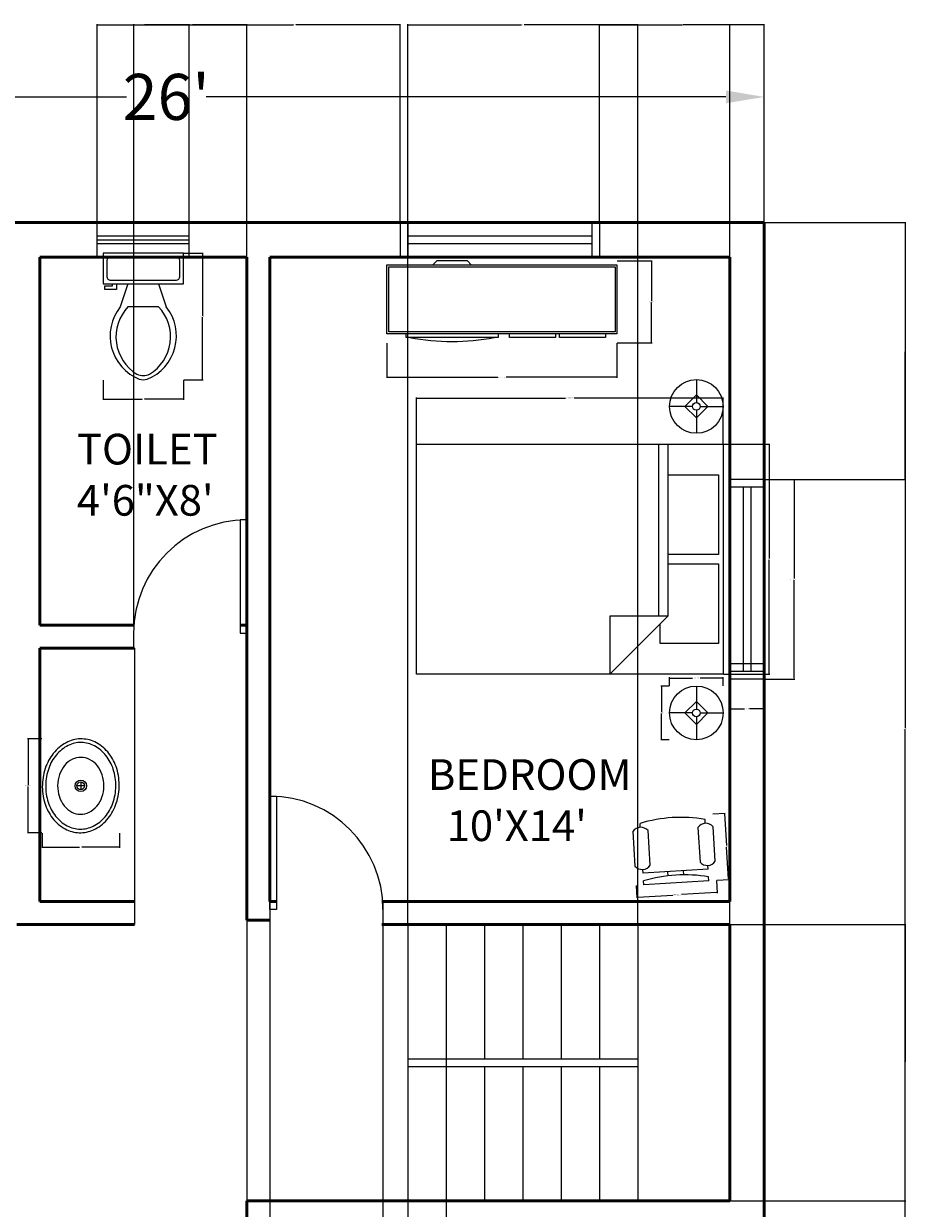
# Model space of a CAD drawing. Units: inches. Extents: x 177 to 602, y 30 to 608.
# Tile 4 of 4: x 372 to 602, y 299 to 608. Entities that reach past the tile are written whole.
import ezdxf

# ---------------------------------------------------------------- set-up
doc = ezdxf.new("R2010")
doc.units = ezdxf.units.IN
doc.header["$MEASUREMENT"] = 0
for name, color, linetype, lineweight in [('A-ANNO-DIMS', 2, 'Continuous', 18), ('A-AREA-IDEN', 7, 'Continuous', 25), ('A-DOOR', 3, 'Continuous', 25), ('A-FLOR-CASE', 32, 'Continuous', 25), ('A-FLOR-FIXT', 9, 'Continuous', 20), ('A-FLOR-STRS', 7, 'Continuous', 25), ('A-FURN', 8, 'Continuous', 18), ('A-GLAZ', 4, 'Continuous', 18), ('A-WALL', 7, 'Continuous', 50)]:
    doc.layers.add(name, color=color, linetype=linetype, lineweight=lineweight)
doc.styles.get("Standard").update_dxf_attribs({"font": 'arial.ttf'})
doc.dimstyles.get("Standard").update_dxf_attribs({"dimtxt": 0.18, "dimasz": 0.18, "dimexe": 0.18, "dimexo": 0.0625, "dimgap": 0.09, "dimtad": 0, "dimtih": 1, "dimtoh": 1, "dimdec": 1, "dimzin": 0, "dimdsep": 46, "dimlunit": 4, "dimtxsty": 'Standard', "dimcen": 0.09, "dimadec": 0, "dimazin": 0, "dimtfac": 1, "dimtdec": 1, "dimtofl": 0, "dimtmove": 0, "dimatfit": 3, "dimfxl": 1, "dimtolj": 1, "dimtzin": 0, "dimarcsym": 0})

# ---------------------------------------------------------------- blocks, each defined once
blk = doc.blocks.new('*U16')
for p, q in [((-750, 0), (-750, -100)), ((0, 0), (0, -100))]:
    blk.add_line(p, q)
blk.add_lwpolyline([(0, 0), (0, 750), (-43.75, 750), (-43.75, 0)], close=True)
blk.add_arc((0, 0), 750, 90, 180)
blk = doc.blocks.new('Toilet - top')
for p, q in [((9.5, -6), (9.5, -2)), ((-10, -8.5), (-8, -8.5)), ((-10, -9.5), (-10, -8.5)), ((-8, -8.5), (-8, -8)), ((-7, -8), (-7, -9.5)), ((-4, -8), (-6, -14)), ((4, -8), (6, -14)), ((-7, -9.5), (-10, -9.5)), ((4, -14), (-4, -14))]:
    blk.add_line(p, q)
blk.add_lwpolyline([(10.5, -8), (10.5, 0), (-10.5, 0), (-10.5, -8)], close=True)
for points in [[(-9.5, -2), (-9.5, -6)], [(8.5, -1), (-8.5, -1)], [(-8.5, -7), (8.5, -7)]]:
    blk.add_lwpolyline(points)
for centre, radius, start, end in [((-8.62, -1.88), 0.884, 81.8699, 188.1301), ((8.62, -1.88), 0.884, 351.8699, 98.1301), ((-8.62, -6.12), 0.884, 171.8699, 278.1301), ((8.62, -6.12), 0.884, 261.8699, 8.1301), ((3.52, -21.58), 12.17, 141.4691, 247.9714), ((4.2, -21.82), 11.33, 136.3677, 238.9468), ((-3.52, -21.58), 12.17, 292.0284, 38.5307), ((-4.2, -21.82), 11.33, 301.053, 43.6321), ((0, -27.88), 4, 245.7318, 294.2682), ((0, -29), 4, 254.8605, 285.1395)]:
    blk.add_arc(centre, radius, start, end)
blk = doc.blocks.new('Sink - Oval top')
for p, q in [((-1, 0), (1, 0)), ((0, 1), (0, -1))]:
    blk.add_line(p, q)
for points in [[(-12.23, 0.39, 0.117634), (-11.46, -3.36, 0.104469), (-8.88, -6.8, 0.090016), (-5.08, -9.07, 0.08192), (-0.32, -10.02, 0.08192), (4.49, -9.38, 0.090016), (8.42, -7.36, 0.104469), (11.22, -4.09, 0.117634), (12.23, -0.39, 0.117634), (11.46, 3.36, 0.104469), (8.88, 6.8, 0.090016), (5.08, 9.07, 0.08192), (0.32, 10.02, 0.08192), (-4.49, 9.38, 0.090016), (-8.42, 7.36, 0.104469), (-11.22, 4.09, 0.117634)], [(-11.29, 0.16, 0.118622), (-10.52, -3.25, 0.104678), (-8.07, -6.36, 0.089562), (-4.54, -8.37, 0.081185), (-0.13, -9.15, 0.081185), (4.3, -8.49, 0.089562), (7.89, -6.58, 0.104678), (10.42, -3.55, 0.118622), (11.29, -0.16, 0.118622), (10.52, 3.25, 0.104678), (8.07, 6.36, 0.089562), (4.54, 8.37, 0.081185), (0.13, 9.15, 0.081185), (-4.3, 8.49, 0.089562), (-7.89, 6.58, 0.104678), (-10.42, 3.55, 0.118622)], [(-7.42, 0.08, 0.118283), (-6.91, -2.17, 0.104607), (-5.29, -4.21, 0.089718), (-2.97, -5.53, 0.081436), (-0.07, -6.04, 0.081436), (2.84, -5.59, 0.089718), (5.2, -4.33, 0.104607), (6.86, -2.32, 0.118283), (7.42, -0.08, 0.118283), (6.91, 2.17, 0.104607), (5.29, 4.21, 0.089718), (2.97, 5.53, 0.081436), (0.07, 6.04, 0.081436), (-2.84, 5.59, 0.089718), (-5.2, 4.33, 0.104607), (-6.86, 2.32, 0.118283)]]:
    blk.add_lwpolyline(points, format="xyb", close=True)
for radius in [1.5, 1]:
    blk.add_circle((0, 0), radius)
blk = doc.blocks.new('*U2')
for p, q in [((0, 0), (0, -100)), ((750, 0), (750, -100))]:
    blk.add_line(p, q)
blk.add_lwpolyline([(0, 0), (0, 750), (43.75, 750), (43.75, 0)], close=True)
blk.add_arc((0, 0), 750, 0, 90)
blk = doc.blocks.new('Bed - Queen')
for p, q in [((0, -80.00003), (0, 0)), ((0, 0), (59.99999, 0)), ((59.99999, 0), (59.99999, -80.00003)), ((7.99999, -1.2), (28.79998, -1.2)), ((7.99999, -14.4), (7.99999, -1.2)), ((28.79998, -1.2), (28.79998, -14.4)), ((31.19999, -1.2), (51.99999, -1.2)), ((31.19999, -14.4), (31.19999, -1.2)), ((51.99999, -1.2), (51.99999, -16.4)), ((0, -14.4), (44.8, -14.4)), ((59.99999, -29.6), (44.8, -14.4)), ((44.8, -14.4), (44.8, -29.6)), ((44.8, -16.8), (0, -16.8)), ((51.99999, -16.4), (46.79936, -16.4)), ((44.8, -29.6), (59.99999, -29.6)), ((59.99999, -80.00003), (0, -80.00003))]:
    blk.add_line(p, q)
blk = doc.blocks.new('Lamp - Table')
for p, q in [((0, 7), (0, 1)), ((-1, 0), (-7, 0)), ((0, 3), (-3, 0)), ((-3, 0), (0, -3)), ((3, 0), (0, 3)), ((0, -3), (3, 0)), ((1, 0), (7, 0)), ((0, -1), (0, -7))]:
    blk.add_line(p, q)
for radius in [7, 1]:
    blk.add_circle((0, 0), radius)
blk = doc.blocks.new('Entertainment Center')
for p, q in [((-4, 0), (-5, -1)), ((4, 0), (-4, 0)), ((5, -1), (4, 0)), ((-17, -19), (-17, -1)), ((-17, -1), (43, -1)), ((-16.5, -18.5), (-16.5, -1.5)), ((-16.5, -1.5), (42.5, -1.5)), ((42.5, -1.5), (42.5, -18.5)), ((43, -1), (43, -19)), ((42.5, -18.5), (-16.5, -18.5)), ((43, -19), (-17, -19)), ((-12, -20), (-12, -19)), ((12, -20), (-12, -20)), ((12, -19), (12, -20)), ((15, -20), (15, -19)), ((27, -20), (15, -20)), ((27, -19), (27, -20)), ((28, -20), (28, -19)), ((40, -20), (28, -20)), ((40, -19), (40, -20))]:
    blk.add_line(p, q)
blk.add_arc((0, 40), 61, 259.6111, 280.3889)
blk = doc.blocks.new('Chair - Desk')
for p, q in [((-8.5, 0), (-8.5, -1)), ((-8.5, 0), (8.5, 0)), ((8.5, 0), (8.5, -1)), ((-8.5, -3), (-8.5, -4)), ((-8.5, -3), (8.5, -3)), ((-2, -3), (-2, -1.9355)), ((2, -1.9576), (2, -3)), ((8.5, -3), (8.5, -4)), ((-10.5, -5), (-10.5, -14)), ((-6.5, -14), (-6.5, -5)), ((6.5, -5), (6.5, -14)), ((10.5, -14), (10.5, -5)), ((-8.5, -15), (-8.5, -16)), ((8.5, -15), (8.5, -16))]:
    blk.add_line(p, q)
for centre, radius, start, end in [((0, 34.625), 36.625, 256.5803, 283.4197), ((-8.5, -6.5), 2.5, 36.8699, 143.1301), ((8.5, -6.5), 2.5, 36.8699, 143.1301), ((-8.5, -12.5), 2.5, 216.8699, 323.1301), ((8.5, -12.5), 2.5, 216.8699, 323.1301), ((0, 19.625), 36.625, 256.5803, 283.4197)]:
    blk.add_arc(centre, radius, start, end)
blk = doc.blocks.new('*D32')
at = {"layer": 'A-ANNO-DIMS', "color": 0, "lineweight": -2, "transparency": 16777216}
for p, q in [((253.34, 556.2), (253.34, 589.06)), ((263.34, 588.88), (398.96, 588.88)), ((555.34, 588.88), (419.71, 588.88)), ((565.34, 556.2), (565.34, 589.06))]:
    blk.add_line(p, q, dxfattribs=at)
at = {"layer": 'A-ANNO-DIMS', "color": 0, "transparency": 16777216}
for points in [[(263.34, 590.55), (263.34, 587.22), (253.34, 588.88)], [(555.34, 590.55), (555.34, 587.22), (565.34, 588.88)]]:
    blk.add_solid(points, dxfattribs=at)
at = {"layer": 'Defpoints', "color": 0, "transparency": 16777216}
for p in [(565.34, 588.88), (253.34, 556.14), (565.34, 556.14)]:
    blk.add_point(p, dxfattribs=at)
at = {"layer": 'A-ANNO-DIMS', "color": 0, "transparency": 16777216, "insert": (409.34, 588.88), "char_height": 12, "attachment_point": 5}
blk.add_mtext("\\A1;26'", dxfattribs=at)
blk = doc.blocks.new('WIN-48IN')
for p, q in [((9, 52), (0, 52)), ((9, 50), (0, 50)), ((3.5, 50), (3.5, 2)), ((5.5, 50), (5.5, 2)), ((9, 2), (0, 2)), ((9, 0), (0, 0))]:
    blk.add_line(p, q)
blk = doc.blocks.new('*D37')
at = {"layer": 'A-ANNO-DIMS', "color": 0, "lineweight": -2, "transparency": 16777216}
for p, q in [((565.4, 489.14), (573.32, 489.14)), ((573.14, 488.96), (573.14, 463.32)), ((573.14, 437.32), (573.14, 462.95)), ((565.4, 437.14), (573.32, 437.14))]:
    blk.add_line(p, q, dxfattribs=at)
at = {"layer": 'A-ANNO-DIMS', "color": 0, "transparency": 16777216}
for points in [[(573.11, 488.96), (573.17, 488.96), (573.14, 489.14)], [(573.11, 437.32), (573.17, 437.32), (573.14, 437.14)]]:
    blk.add_solid(points, dxfattribs=at)
at = {"layer": 'Defpoints', "color": 0, "transparency": 16777216}
for p in [(565.34, 489.14), (573.14, 489.14), (565.34, 437.14)]:
    blk.add_point(p, dxfattribs=at)
at = {"layer": 'A-ANNO-DIMS', "color": 0, "transparency": 16777216, "insert": (573.14, 463.14), "char_height": 0.18, "attachment_point": 5}
blk.add_mtext('\\A1;WINDOW 4\'-4" TYP.', dxfattribs=at)
blk = doc.blocks.new('*D38')
at = {"layer": 'A-ANNO-DIMS', "color": 0, "lineweight": -2, "transparency": 16777216}
for p, q in [((556.34, 437.07), (556.34, 429.16)), ((565.34, 437.07), (565.34, 429.16)), ((556.52, 429.34), (560.2, 429.34)), ((565.16, 429.34), (561.48, 429.34))]:
    blk.add_line(p, q, dxfattribs=at)
at = {"layer": 'A-ANNO-DIMS', "color": 0, "transparency": 16777216}
for points in [[(556.52, 429.37), (556.52, 429.31), (556.34, 429.34)], [(565.16, 429.37), (565.16, 429.31), (565.34, 429.34)]]:
    blk.add_solid(points, dxfattribs=at)
at = {"layer": 'Defpoints', "color": 0, "transparency": 16777216}
for p in [(556.34, 437.14), (565.34, 437.14), (565.34, 429.34)]:
    blk.add_point(p, dxfattribs=at)
at = {"layer": 'A-ANNO-DIMS', "color": 0, "transparency": 16777216, "insert": (560.84, 429.34), "char_height": 0.18, "attachment_point": 5}
blk.add_mtext('\\A1;0\'-9" TYP.', dxfattribs=at)
blk = doc.blocks.new('*D39')
at = {"layer": 'A-ANNO-DIMS', "color": 0, "lineweight": -2, "transparency": 16777216}
for p, q in [((540.61, 435.37), (540.61, 437.58)), ((540.79, 437.4), (546.6, 437.4)), ((554.43, 437.4), (548.62, 437.4)), ((554.61, 435.37), (554.61, 437.58))]:
    blk.add_line(p, q, dxfattribs=at)
at = {"layer": 'A-ANNO-DIMS', "color": 0, "transparency": 16777216}
for points in [[(540.79, 437.43), (540.79, 437.37), (540.61, 437.4)], [(554.43, 437.43), (554.43, 437.37), (554.61, 437.4)]]:
    blk.add_solid(points, dxfattribs=at)
at = {"layer": 'Defpoints', "color": 0, "transparency": 16777216}
for p in [(554.61, 437.4), (540.61, 435.3), (554.61, 435.3)]:
    blk.add_point(p, dxfattribs=at)
at = {"layer": 'A-ANNO-DIMS', "color": 0, "transparency": 16777216, "insert": (547.61, 437.4), "char_height": 0.18, "attachment_point": 5}
blk.add_mtext('\\A1;LAMP 1\'-2" TYP.', dxfattribs=at)
blk = doc.blocks.new('*D40')
at = {"layer": 'A-ANNO-DIMS', "color": 0, "lineweight": -2, "transparency": 16777216}
for p, q in [((540.55, 435.3), (538.33, 435.3)), ((538.51, 435.12), (538.51, 428.48)), ((538.51, 421.48), (538.51, 428.12)), ((540.55, 421.3), (538.33, 421.3))]:
    blk.add_line(p, q, dxfattribs=at)
at = {"layer": 'A-ANNO-DIMS', "color": 0, "transparency": 16777216}
for points in [[(538.48, 435.12), (538.54, 435.12), (538.51, 435.3)], [(538.48, 421.48), (538.54, 421.48), (538.51, 421.3)]]:
    blk.add_solid(points, dxfattribs=at)
at = {"layer": 'Defpoints', "color": 0, "transparency": 16777216}
for p in [(538.51, 435.3), (540.61, 435.3), (540.61, 421.3)]:
    blk.add_point(p, dxfattribs=at)
at = {"layer": 'A-ANNO-DIMS', "color": 0, "transparency": 16777216, "insert": (538.51, 428.3), "char_height": 0.18, "attachment_point": 5}
blk.add_mtext('\\A1;1\'-2" TYP.', dxfattribs=at)
blk = doc.blocks.new('*D49')
at = {"layer": 'A-ANNO-DIMS', "color": 0, "lineweight": -2, "transparency": 16777216}
for p, q in [((413.9, 548.14), (418.98, 548.14)), ((418.8, 547.96), (418.8, 531.8)), ((418.8, 515.27), (418.8, 531.43)), ((413.9, 515.09), (418.98, 515.09))]:
    blk.add_line(p, q, dxfattribs=at)
at = {"layer": 'A-ANNO-DIMS', "color": 0, "transparency": 16777216}
for points in [[(418.77, 547.96), (418.83, 547.96), (418.8, 548.14)], [(418.77, 515.27), (418.83, 515.27), (418.8, 515.09)]]:
    blk.add_solid(points, dxfattribs=at)
at = {"layer": 'Defpoints', "color": 0, "transparency": 16777216}
for p in [(413.84, 548.14), (418.8, 548.14), (413.84, 515.09)]:
    blk.add_point(p, dxfattribs=at)
at = {"layer": 'A-ANNO-DIMS', "color": 0, "transparency": 16777216, "insert": (418.8, 531.61), "char_height": 0.18, "attachment_point": 5}
blk.add_mtext('\\A1;WC 2\'-9"', dxfattribs=at)
blk = doc.blocks.new('*D50')
at = {"layer": 'A-ANNO-DIMS', "color": 0, "lineweight": -2, "transparency": 16777216}
for p, q in [((392.84, 515.03), (392.84, 509.95)), ((413.84, 515.03), (413.84, 509.95)), ((393.02, 510.13), (403.02, 510.13)), ((413.66, 510.13), (403.66, 510.13))]:
    blk.add_line(p, q, dxfattribs=at)
at = {"layer": 'A-ANNO-DIMS', "color": 0, "transparency": 16777216}
for points in [[(393.02, 510.16), (393.02, 510.1), (392.84, 510.13)], [(413.66, 510.16), (413.66, 510.1), (413.84, 510.13)]]:
    blk.add_solid(points, dxfattribs=at)
at = {"layer": 'Defpoints', "color": 0, "transparency": 16777216}
for p in [(392.84, 515.09), (413.84, 515.09), (413.84, 510.13)]:
    blk.add_point(p, dxfattribs=at)
at = {"layer": 'A-ANNO-DIMS', "color": 0, "transparency": 16777216, "insert": (403.34, 510.13), "char_height": 0.18, "attachment_point": 5}
blk.add_mtext('\\A1;1\'-9"', dxfattribs=at)
blk = doc.blocks.new('*D51')
at = {"layer": 'A-ANNO-DIMS', "color": 0, "lineweight": -2, "transparency": 16777216}
for p, q in [((376.9, 421.58), (373.1, 421.58)), ((373.28, 421.4), (373.28, 409.48)), ((373.28, 397.21), (373.28, 409.12)), ((376.9, 397.03), (373.1, 397.03))]:
    blk.add_line(p, q, dxfattribs=at)
at = {"layer": 'A-ANNO-DIMS', "color": 0, "transparency": 16777216}
for points in [[(373.25, 421.4), (373.31, 421.4), (373.28, 421.58)], [(373.25, 397.21), (373.31, 397.21), (373.28, 397.03)]]:
    blk.add_solid(points, dxfattribs=at)
at = {"layer": 'Defpoints', "color": 0, "transparency": 16777216}
for p in [(376.96, 421.58), (373.28, 397.03), (376.96, 397.03)]:
    blk.add_point(p, dxfattribs=at)
at = {"layer": 'A-ANNO-DIMS', "color": 0, "transparency": 16777216, "insert": (373.28, 409.3), "char_height": 0.18, "attachment_point": 5}
blk.add_mtext('\\A1;BASIN 2\'-0 1/2"', dxfattribs=at)
blk = doc.blocks.new('*D52')
at = {"layer": 'A-ANNO-DIMS', "color": 0, "lineweight": -2, "transparency": 16777216}
for p, q in [((376.96, 396.96), (376.96, 393.16)), ((397.1, 396.96), (397.1, 393.16)), ((377.14, 393.34), (386.71, 393.34)), ((396.92, 393.34), (387.35, 393.34))]:
    blk.add_line(p, q, dxfattribs=at)
at = {"layer": 'A-ANNO-DIMS', "color": 0, "transparency": 16777216}
for points in [[(377.14, 393.37), (377.14, 393.31), (376.96, 393.34)], [(396.92, 393.37), (396.92, 393.31), (397.1, 393.34)]]:
    blk.add_solid(points, dxfattribs=at)
at = {"layer": 'Defpoints', "color": 0, "transparency": 16777216}
for p in [(376.96, 397.03), (397.1, 397.03), (397.1, 393.34)]:
    blk.add_point(p, dxfattribs=at)
at = {"layer": 'A-ANNO-DIMS', "color": 0, "transparency": 16777216, "insert": (387.03, 393.34), "char_height": 0.18, "attachment_point": 5}
blk.add_mtext('\\A1;1\'-8"', dxfattribs=at)
blk = doc.blocks.new('*D53')
at = {"layer": 'A-ANNO-DIMS', "color": 0, "lineweight": -2, "transparency": 16777216}
for p, q in [((474.61, 498.42), (474.61, 510.54)), ((474.79, 510.36), (513.5, 510.36)), ((554.43, 510.36), (515.71, 510.36)), ((554.61, 498.42), (554.61, 510.54))]:
    blk.add_line(p, q, dxfattribs=at)
at = {"layer": 'A-ANNO-DIMS', "color": 0, "transparency": 16777216}
for points in [[(474.79, 510.39), (474.79, 510.33), (474.61, 510.36)], [(554.43, 510.39), (554.43, 510.33), (554.61, 510.36)]]:
    blk.add_solid(points, dxfattribs=at)
at = {"layer": 'Defpoints', "color": 0, "transparency": 16777216}
for p in [(554.61, 510.36), (474.61, 498.36), (554.61, 498.36)]:
    blk.add_point(p, dxfattribs=at)
at = {"layer": 'A-ANNO-DIMS', "color": 0, "transparency": 16777216, "insert": (514.61, 510.36), "char_height": 0.18, "attachment_point": 5}
blk.add_mtext('\\A1;QUEEN BED 6\'-8"', dxfattribs=at)
blk = doc.blocks.new('*D54')
at = {"layer": 'A-ANNO-DIMS', "color": 0, "lineweight": -2, "transparency": 16777216}
for p, q in [((554.67, 498.36), (566.79, 498.36)), ((566.61, 498.18), (566.61, 468.54)), ((566.61, 438.54), (566.61, 468.18)), ((554.67, 438.36), (566.79, 438.36))]:
    blk.add_line(p, q, dxfattribs=at)
at = {"layer": 'A-ANNO-DIMS', "color": 0, "transparency": 16777216}
for points in [[(566.58, 498.18), (566.64, 498.18), (566.61, 498.36)], [(566.58, 438.54), (566.64, 438.54), (566.61, 438.36)]]:
    blk.add_solid(points, dxfattribs=at)
at = {"layer": 'Defpoints', "color": 0, "transparency": 16777216}
for p in [(554.61, 498.36), (554.61, 438.36), (566.61, 438.36)]:
    blk.add_point(p, dxfattribs=at)
at = {"layer": 'A-ANNO-DIMS', "color": 0, "transparency": 16777216, "insert": (566.61, 468.36), "char_height": 0.18, "attachment_point": 5}
blk.add_mtext('\\A1;5\'-0"', dxfattribs=at)
blk = doc.blocks.new('*D55')
at = {"layer": 'A-ANNO-DIMS', "color": 0, "lineweight": -2, "transparency": 16777216}
for p, q in [((466.89, 524.73), (466.89, 515.61)), ((526.89, 524.73), (526.89, 515.61)), ((467.07, 515.79), (495.81, 515.79)), ((526.71, 515.79), (497.98, 515.79))]:
    blk.add_line(p, q, dxfattribs=at)
at = {"layer": 'A-ANNO-DIMS', "color": 0, "transparency": 16777216}
for points in [[(467.07, 515.82), (467.07, 515.76), (466.89, 515.79)], [(526.71, 515.82), (526.71, 515.76), (526.89, 515.79)]]:
    blk.add_solid(points, dxfattribs=at)
at = {"layer": 'Defpoints', "color": 0, "transparency": 16777216}
for p in [(466.89, 524.79), (526.89, 524.79), (526.89, 515.79)]:
    blk.add_point(p, dxfattribs=at)
at = {"layer": 'A-ANNO-DIMS', "color": 0, "transparency": 16777216, "insert": (496.89, 515.79), "char_height": 0.18, "attachment_point": 5}
blk.add_mtext('\\A1;MEDIA UNIT 5\'-0"', dxfattribs=at)
blk = doc.blocks.new('*D56')
at = {"layer": 'A-ANNO-DIMS', "color": 0, "lineweight": -2, "transparency": 16777216}
for p, q in [((526.96, 546.13), (536.07, 546.13)), ((535.89, 545.95), (535.89, 535.64)), ((535.89, 524.97), (535.89, 535.28)), ((526.96, 524.79), (536.07, 524.79))]:
    blk.add_line(p, q, dxfattribs=at)
at = {"layer": 'A-ANNO-DIMS', "color": 0, "transparency": 16777216}
for points in [[(535.86, 545.95), (535.92, 545.95), (535.89, 546.13)], [(535.86, 524.97), (535.92, 524.97), (535.89, 524.79)]]:
    blk.add_solid(points, dxfattribs=at)
at = {"layer": 'Defpoints', "color": 0, "transparency": 16777216}
for p in [(526.89, 546.13), (535.89, 546.13), (526.89, 524.79)]:
    blk.add_point(p, dxfattribs=at)
at = {"layer": 'A-ANNO-DIMS', "color": 0, "transparency": 16777216, "insert": (535.89, 535.46), "char_height": 0.18, "attachment_point": 5}
blk.add_mtext('\\A1;1\'-9 1/2"', dxfattribs=at)
blk = doc.blocks.new('*D63')
at = {"layer": 'A-ANNO-DIMS', "color": 0, "lineweight": -2, "transparency": 16777216}
for p, q in [((531.91, 383.32), (532.11, 380.06)), ((552.87, 384.61), (553.07, 381.35)), ((532.28, 380.25), (541.45, 380.82)), ((552.88, 381.52), (543.7, 380.95))]:
    blk.add_line(p, q, dxfattribs=at)
at = {"layer": 'A-ANNO-DIMS', "color": 0, "transparency": 16777216}
for points in [[(532.27, 380.28), (532.28, 380.22), (532.1, 380.24)], [(552.88, 381.55), (552.88, 381.49), (553.06, 381.53)]]:
    blk.add_solid(points, dxfattribs=at)
at = {"layer": 'Defpoints', "color": 0, "transparency": 16777216}
for p in [(531.9, 383.39), (552.86, 384.67), (532.1, 380.24)]:
    blk.add_point(p, dxfattribs=at)
at = {"layer": 'A-ANNO-DIMS', "color": 0, "transparency": 16777216, "insert": (542.58, 380.88), "char_height": 0.18, "attachment_point": 5}
blk.add_mtext('\\A1;DESK CHAIR 1\'-9"', dxfattribs=at)
blk = doc.blocks.new('*D64')
at = {"layer": 'A-ANNO-DIMS', "color": 0, "lineweight": -2, "transparency": 16777216}
for p, q in [((551.87, 401.98), (555.13, 402.18)), ((554.96, 401.98), (555.47, 393.7)), ((556, 385.04), (555.49, 393.33)), ((552.93, 384.67), (556.19, 384.87))]:
    blk.add_line(p, q, dxfattribs=at)
at = {"layer": 'A-ANNO-DIMS', "color": 0, "transparency": 16777216}
for points in [[(554.99, 401.99), (554.93, 401.98), (554.95, 402.16)], [(556.03, 385.04), (555.97, 385.04), (556.01, 384.86)]]:
    blk.add_solid(points, dxfattribs=at)
at = {"layer": 'Defpoints', "color": 0, "transparency": 16777216}
for p in [(551.8, 401.97), (552.86, 384.67), (556.01, 384.86)]:
    blk.add_point(p, dxfattribs=at)
at = {"layer": 'A-ANNO-DIMS', "color": 0, "transparency": 16777216, "insert": (555.48, 393.51), "char_height": 0.18, "attachment_point": 5}
blk.add_mtext('\\A1;1\'-5 1/2"', dxfattribs=at)
blk = doc.blocks.new('*D74')
at = {"layer": 'A-ANNO-DIMS', "color": 0, "lineweight": -2, "transparency": 16777216}
for p, q in [((565.4, 556.14), (602.22, 556.14)), ((602.04, 555.96), (602.04, 424.32)), ((602.04, 292.32), (602.04, 423.96)), ((565.4, 292.14), (602.22, 292.14))]:
    blk.add_line(p, q, dxfattribs=at)
at = {"layer": 'A-ANNO-DIMS', "color": 0, "transparency": 16777216}
for points in [[(602.01, 555.96), (602.07, 555.96), (602.04, 556.14)], [(602.01, 292.32), (602.07, 292.32), (602.04, 292.14)]]:
    blk.add_solid(points, dxfattribs=at)
at = {"layer": 'Defpoints', "color": 0, "transparency": 16777216}
for p in [(565.34, 556.14), (602.04, 556.14), (565.34, 292.14)]:
    blk.add_point(p, dxfattribs=at)
at = {"layer": 'A-ANNO-DIMS', "color": 0, "transparency": 16777216, "insert": (602.04, 424.14), "char_height": 0.18, "attachment_point": 5}
blk.add_mtext('\\A1;22\'-0"', dxfattribs=at)
blk = doc.blocks.new('*D79')
at = {"layer": 'A-ANNO-DIMS', "color": 0, "lineweight": -2, "transparency": 16777216}
for p, q in [((522.34, 556.2), (522.34, 607.88)), ((522.52, 607.7), (543.51, 607.7)), ((565.16, 607.7), (544.17, 607.7)), ((565.34, 556.2), (565.34, 607.88))]:
    blk.add_line(p, q, dxfattribs=at)
at = {"layer": 'A-ANNO-DIMS', "color": 0, "transparency": 16777216}
for points in [[(522.52, 607.73), (522.52, 607.67), (522.34, 607.7)], [(565.16, 607.73), (565.16, 607.67), (565.34, 607.7)]]:
    blk.add_solid(points, dxfattribs=at)
at = {"layer": 'Defpoints', "color": 0, "transparency": 16777216}
for p in [(565.34, 607.7), (522.34, 556.14), (565.34, 556.14)]:
    blk.add_point(p, dxfattribs=at)
at = {"layer": 'A-ANNO-DIMS', "color": 0, "transparency": 16777216, "insert": (543.84, 607.7), "char_height": 0.18, "attachment_point": 5}
blk.add_mtext('\\A1;3\'-7"', dxfattribs=at)
blk = doc.blocks.new('*D80')
at = {"layer": 'A-ANNO-DIMS', "color": 0, "lineweight": -2, "transparency": 16777216}
for p, q in [((565.4, 556.14), (602.22, 556.14)), ((602.04, 555.96), (602.04, 522.82)), ((602.04, 489.32), (602.04, 522.46)), ((565.4, 489.14), (602.22, 489.14))]:
    blk.add_line(p, q, dxfattribs=at)
at = {"layer": 'A-ANNO-DIMS', "color": 0, "transparency": 16777216}
for points in [[(602.01, 555.96), (602.07, 555.96), (602.04, 556.14)], [(602.01, 489.32), (602.07, 489.32), (602.04, 489.14)]]:
    blk.add_solid(points, dxfattribs=at)
at = {"layer": 'Defpoints', "color": 0, "transparency": 16777216}
for p in [(565.34, 556.14), (602.04, 556.14), (565.34, 489.14)]:
    blk.add_point(p, dxfattribs=at)
at = {"layer": 'A-ANNO-DIMS', "color": 0, "transparency": 16777216, "insert": (602.04, 522.64), "char_height": 0.18, "attachment_point": 5}
blk.add_mtext('\\A1;5\'-7"', dxfattribs=at)
blk = doc.blocks.new('*D82')
at = {"layer": 'A-ANNO-DIMS', "color": 0, "lineweight": -2, "transparency": 16777216}
for p, q in [((391.34, 556.2), (391.34, 607.88)), ((391.52, 607.7), (403.01, 607.7)), ((415.16, 607.7), (403.67, 607.7)), ((415.34, 556.2), (415.34, 607.88))]:
    blk.add_line(p, q, dxfattribs=at)
at = {"layer": 'A-ANNO-DIMS', "color": 0, "transparency": 16777216}
for points in [[(391.52, 607.73), (391.52, 607.67), (391.34, 607.7)], [(415.16, 607.73), (415.16, 607.67), (415.34, 607.7)]]:
    blk.add_solid(points, dxfattribs=at)
at = {"layer": 'Defpoints', "color": 0, "transparency": 16777216}
for p in [(415.34, 607.7), (391.34, 556.14), (415.34, 556.14)]:
    blk.add_point(p, dxfattribs=at)
at = {"layer": 'A-ANNO-DIMS', "color": 0, "transparency": 16777216, "insert": (403.34, 607.7), "char_height": 0.18, "attachment_point": 5}
blk.add_mtext('\\A1;2\'-0"', dxfattribs=at)
blk = doc.blocks.new('*D83')
at = {"layer": 'A-ANNO-DIMS', "color": 0, "lineweight": -2, "transparency": 16777216}
for p, q in [((415.34, 556.2), (415.34, 607.88)), ((415.52, 607.7), (442.51, 607.7)), ((470.16, 607.7), (443.17, 607.7)), ((470.34, 556.2), (470.34, 607.88))]:
    blk.add_line(p, q, dxfattribs=at)
at = {"layer": 'A-ANNO-DIMS', "color": 0, "transparency": 16777216}
for points in [[(415.52, 607.73), (415.52, 607.67), (415.34, 607.7)], [(470.16, 607.73), (470.16, 607.67), (470.34, 607.7)]]:
    blk.add_solid(points, dxfattribs=at)
at = {"layer": 'Defpoints', "color": 0, "transparency": 16777216}
for p in [(470.34, 607.7), (415.34, 556.14), (470.34, 556.14)]:
    blk.add_point(p, dxfattribs=at)
at = {"layer": 'A-ANNO-DIMS', "color": 0, "transparency": 16777216, "insert": (442.84, 607.7), "char_height": 0.18, "attachment_point": 5}
blk.add_mtext('\\A1;4\'-7"', dxfattribs=at)
blk = doc.blocks.new('*D84')
at = {"layer": 'A-ANNO-DIMS', "color": 0, "lineweight": -2, "transparency": 16777216}
for p, q in [((436.34, 379.07), (436.34, 30.54)), ((430.34, 374.22), (430.34, 30.54)), ((430.52, 30.72), (433.01, 30.72)), ((436.16, 30.72), (433.67, 30.72))]:
    blk.add_line(p, q, dxfattribs=at)
at = {"layer": 'A-ANNO-DIMS', "color": 0, "transparency": 16777216}
for points in [[(430.52, 30.75), (430.52, 30.69), (430.34, 30.72)], [(436.16, 30.75), (436.16, 30.69), (436.34, 30.72)]]:
    blk.add_solid(points, dxfattribs=at)
at = {"layer": 'Defpoints', "color": 0, "transparency": 16777216}
for p in [(436.34, 379.14), (430.34, 374.28), (430.34, 30.72)]:
    blk.add_point(p, dxfattribs=at)
at = {"layer": 'A-ANNO-DIMS', "color": 0, "transparency": 16777216, "insert": (433.34, 30.72), "char_height": 0.18, "attachment_point": 5}
blk.add_mtext('\\A1;0\'-6"', dxfattribs=at)
blk = doc.blocks.new('*D87')
at = {"layer": 'A-ANNO-DIMS', "color": 0, "lineweight": -2, "transparency": 16777216}
for p, q in [((436.34, 379.07), (436.34, 30.54)), ((465.79, 379.07), (465.79, 30.54)), ((436.52, 30.72), (450.53, 30.72)), ((465.61, 30.72), (451.61, 30.72))]:
    blk.add_line(p, q, dxfattribs=at)
at = {"layer": 'A-ANNO-DIMS', "color": 0, "transparency": 16777216}
for points in [[(436.52, 30.75), (436.52, 30.69), (436.34, 30.72)], [(465.61, 30.75), (465.61, 30.69), (465.79, 30.72)]]:
    blk.add_solid(points, dxfattribs=at)
at = {"layer": 'Defpoints', "color": 0, "transparency": 16777216}
for p in [(436.34, 379.14), (465.79, 379.14), (465.79, 30.72)]:
    blk.add_point(p, dxfattribs=at)
at = {"layer": 'A-ANNO-DIMS', "color": 0, "transparency": 16777216, "insert": (451.07, 30.72), "char_height": 0.18, "attachment_point": 5}
blk.add_mtext('\\A1;2\'-5 1/2"', dxfattribs=at)
blk = doc.blocks.new('*D88')
at = {"layer": 'A-ANNO-DIMS', "color": 0, "lineweight": -2, "transparency": 16777216}
for p, q in [((400.88, 451.2), (400.88, 607.88)), ((401.06, 607.7), (415.07, 607.7)), ((430.16, 607.7), (416.15, 607.7)), ((430.34, 451.2), (430.34, 607.88))]:
    blk.add_line(p, q, dxfattribs=at)
at = {"layer": 'A-ANNO-DIMS', "color": 0, "transparency": 16777216}
for points in [[(401.06, 607.73), (401.06, 607.67), (400.88, 607.7)], [(430.16, 607.73), (430.16, 607.67), (430.34, 607.7)]]:
    blk.add_solid(points, dxfattribs=at)
at = {"layer": 'Defpoints', "color": 0, "transparency": 16777216}
for p in [(430.34, 607.7), (400.88, 451.14), (430.34, 451.14)]:
    blk.add_point(p, dxfattribs=at)
at = {"layer": 'A-ANNO-DIMS', "color": 0, "transparency": 16777216, "insert": (415.61, 607.7), "char_height": 0.18, "attachment_point": 5}
blk.add_mtext('\\A1;2\'-5 1/2"', dxfattribs=at)
blk = doc.blocks.new('*D89')
at = {"layer": 'A-ANNO-DIMS', "color": 0, "lineweight": -2, "transparency": 16777216}
for p, q in [((556.4, 373.14), (602.22, 373.14)), ((602.04, 372.96), (602.04, 337.32)), ((602.04, 301.32), (602.04, 336.96)), ((556.4, 301.14), (602.22, 301.14))]:
    blk.add_line(p, q, dxfattribs=at)
at = {"layer": 'A-ANNO-DIMS', "color": 0, "transparency": 16777216}
for points in [[(602.01, 372.96), (602.07, 372.96), (602.04, 373.14)], [(602.01, 301.32), (602.07, 301.32), (602.04, 301.14)]]:
    blk.add_solid(points, dxfattribs=at)
at = {"layer": 'Defpoints', "color": 0, "transparency": 16777216}
for p in [(556.34, 373.14), (602.04, 373.14), (556.34, 301.14)]:
    blk.add_point(p, dxfattribs=at)
at = {"layer": 'A-ANNO-DIMS', "color": 0, "transparency": 16777216, "insert": (602.04, 337.14), "char_height": 0.18, "attachment_point": 5}
blk.add_mtext('\\A1;6\'-0"', dxfattribs=at)
blk = doc.blocks.new('*D90')
at = {"layer": 'A-ANNO-DIMS', "color": 0, "lineweight": -2, "transparency": 16777216}
for p, q in [((472.34, 373.2), (472.34, 607.88)), ((472.52, 607.7), (502.01, 607.7)), ((532.16, 607.7), (502.67, 607.7)), ((532.34, 373.2), (532.34, 607.88))]:
    blk.add_line(p, q, dxfattribs=at)
at = {"layer": 'A-ANNO-DIMS', "color": 0, "transparency": 16777216}
for points in [[(472.52, 607.73), (472.52, 607.67), (472.34, 607.7)], [(532.16, 607.73), (532.16, 607.67), (532.34, 607.7)]]:
    blk.add_solid(points, dxfattribs=at)
at = {"layer": 'Defpoints', "color": 0, "transparency": 16777216}
for p in [(532.34, 607.7), (472.34, 373.14), (532.34, 373.14)]:
    blk.add_point(p, dxfattribs=at)
at = {"layer": 'A-ANNO-DIMS', "color": 0, "transparency": 16777216, "insert": (502.34, 607.7), "char_height": 0.18, "attachment_point": 5}
blk.add_mtext('\\A1;5\'-0"', dxfattribs=at)
blk = doc.blocks.new('*D91')
at = {"layer": 'A-ANNO-DIMS', "color": 0, "lineweight": -2, "transparency": 16777216}
for p, q in [((532.34, 373.2), (532.34, 607.88)), ((532.52, 607.7), (544.01, 607.7)), ((556.16, 607.7), (544.67, 607.7)), ((556.34, 373.2), (556.34, 607.88))]:
    blk.add_line(p, q, dxfattribs=at)
at = {"layer": 'A-ANNO-DIMS', "color": 0, "transparency": 16777216}
for points in [[(532.52, 607.73), (532.52, 607.67), (532.34, 607.7)], [(556.16, 607.73), (556.16, 607.67), (556.34, 607.7)]]:
    blk.add_solid(points, dxfattribs=at)
at = {"layer": 'Defpoints', "color": 0, "transparency": 16777216}
for p in [(556.34, 607.7), (532.34, 373.14), (556.34, 373.14)]:
    blk.add_point(p, dxfattribs=at)
at = {"layer": 'A-ANNO-DIMS', "color": 0, "transparency": 16777216, "insert": (544.34, 607.7), "char_height": 0.18, "attachment_point": 5}
blk.add_mtext('\\A1;2\'-0"', dxfattribs=at)
blk = doc.blocks.new('*D92')
at = {"layer": 'A-ANNO-DIMS', "color": 0, "lineweight": -2, "transparency": 16777216}
for p, q in [((472.34, 373.07), (472.34, 30.54)), ((482.34, 373.07), (482.34, 30.54)), ((472.52, 30.72), (476.94, 30.72)), ((482.16, 30.72), (477.74, 30.72))]:
    blk.add_line(p, q, dxfattribs=at)
at = {"layer": 'A-ANNO-DIMS', "color": 0, "transparency": 16777216}
for points in [[(472.52, 30.75), (472.52, 30.69), (472.34, 30.72)], [(482.16, 30.75), (482.16, 30.69), (482.34, 30.72)]]:
    blk.add_solid(points, dxfattribs=at)
at = {"layer": 'Defpoints', "color": 0, "transparency": 16777216}
for p in [(472.34, 373.14), (482.34, 373.14), (482.34, 30.72)]:
    blk.add_point(p, dxfattribs=at)
at = {"layer": 'A-ANNO-DIMS', "color": 0, "transparency": 16777216, "insert": (477.34, 30.72), "char_height": 0.18, "attachment_point": 5}
blk.add_mtext('\\A1;0\'-10"', dxfattribs=at)

msp = doc.modelspace()

# ---------------------------------------------------------------- linework, layer by layer
at = {"layer": 'A-FLOR-CASE'}
msp.add_line((401.08, 445.14), (401.08, 373.14), dxfattribs=at)
at = {"layer": 'A-FLOR-STRS'}
for p, q in [((472.34, 373.14), (472.34, 301.14)), ((482.34, 373.14), (482.34, 338.14)), ((492.34, 373.14), (492.34, 338.14)), ((502.34, 373.14), (502.34, 338.14)), ((512.34, 373.14), (512.34, 338.14)), ((522.34, 373.14), (522.34, 338.14)), ((532.34, 373.14), (532.34, 301.14)), ((472.34, 338.14), (532.34, 338.14)), ((472.34, 336.14), (532.34, 336.14)), ((482.34, 336.14), (482.34, 301.14)), ((492.34, 336.14), (492.34, 301.14)), ((502.34, 336.14), (502.34, 301.14)), ((512.34, 336.14), (512.34, 301.14)), ((522.34, 336.14), (522.34, 301.14))]:
    msp.add_line(p, q, dxfattribs=at)
at = {"layer": 'A-GLAZ'}
for p, q in [((391.34, 547.14), (391.34, 556.14)), ((415.34, 547.14), (415.34, 556.14)), ((391.34, 552.64), (415.34, 552.64)), ((391.34, 551.64), (415.34, 551.64)), ((391.34, 550.64), (415.34, 550.64)), ((556.34, 441.14), (565.34, 441.14))]:
    msp.add_line(p, q, dxfattribs=at)
at = {"layer": 'A-WALL'}
for p, q in [((333.43, 556.14), (565.34, 556.14)), ((565.34, 556.14), (565.34, 292.14)), ((376.34, 547.14), (430.34, 547.14)), ((376.34, 451.14), (376.34, 547.14)), ((430.34, 374.28), (430.34, 547.14)), ((436.34, 547.14), (556.34, 547.14)), ((436.34, 379.14), (436.34, 547.14)), ((556.34, 547.14), (556.34, 379.14)), ((556.34, 451.14), (556.34, 547.14)), ((376.34, 451.14), (400.88, 451.14)), ((428.62, 451.14), (430.34, 451.14)), ((376.34, 379.14), (376.34, 445.14)), ((376.34, 445.14), (401.08, 445.14)), ((376.34, 379.14), (401.08, 379.14)), ((436.34, 379.14), (438.06, 379.14)), ((465.79, 379.14), (556.34, 379.14)), ((430.34, 374.28), (436.34, 374.28)), ((370.34, 373.14), (401.08, 373.14)), ((465.6, 373.14), (556.34, 373.14)), ((556.34, 373.14), (556.34, 301.14)), ((430.34, 292.14), (430.34, 301.14)), ((430.34, 301.14), (556.34, 301.14))]:
    msp.add_line(p, q, dxfattribs=at)

# ---------------------------------------------------------------- block references
at = {"layer": 'A-DOOR', "xscale": 0.0393700787401575, "yscale": 0.0393700787401575, "zscale": 0.0393700787401575}
for name, p in [('*U16', (430.34, 449.07)), ('*U2', (436.34, 377.07))]:
    msp.add_blockref(name, p, dxfattribs=at)
at = {"layer": 'A-FLOR-FIXT'}
msp.add_blockref('Toilet - top', (403.34, 548.14), dxfattribs=at)
at = {"layer": 'A-FLOR-FIXT', "rotation": 270}
msp.add_blockref('Sink - Oval top', (387.03, 409.3), dxfattribs=at)
at = {"layer": 'A-FURN'}
for name, p in [('Entertainment Center', (483.89, 546.13)), ('Lamp - Table', (547.61, 508.19)), ('Lamp - Table', (547.61, 428.3))]:
    msp.add_blockref(name, p, dxfattribs=at)
for name, p, rotation in [('Bed - Queen', (554.61, 498.36), 270), ('Chair - Desk', (542.38, 384.03), 183.5058802023621)]:
    msp.add_blockref(name, p, dxfattribs=dict(at, rotation=rotation))
at = {"layer": 'A-GLAZ', "rotation": 89.99999999999991}
msp.add_blockref('WIN-48IN', (522.34, 547.14), dxfattribs=at)
at = {"layer": 'A-GLAZ'}
msp.add_blockref('WIN-48IN', (556.34, 437.14), dxfattribs=at)

# ---------------------------------------------------------------- texts
at = {"layer": 'A-AREA-IDEN', "char_height": 8, "attachment_point": 1}
for s, insert in [('TOILET\\P4\'6"X8\'', (386.02, 501.06)), ("BEDROOM\\P  10'X14'", (477.59, 416.23)), ('  LIVING\\P19\'6"X12\'1"', (330.54, 305.6))]:
    msp.add_mtext_dynamic_manual_height_columns(s, width=62.7486, gutter_width=1, heights=[0], dxfattribs=dict(at, insert=insert))

# ---------------------------------------------------------------- dimensions: what is measured, and where the dimension line sits
at = {"layer": 'A-ANNO-DIMS'}
for base, p1, p2, override, picture, middle in [((415.34, 607.7), (391.34, 556.14), (415.34, 556.14), {"dimdec": 1, "dimlfac": 1, "dimrnd": 0, "dimzin": 1, "dimdsep": 46, "dimlunit": 4, "dimfrac": 2}, '*D82', (403.34, 607.7)), ((430.34, 607.7), (400.88, 451.14), (430.34, 451.14), {"dimdec": 1, "dimlfac": 1, "dimrnd": 0, "dimzin": 1, "dimdsep": 46, "dimlunit": 4, "dimfrac": 2}, '*D88', (415.61, 607.7)), ((470.34, 607.7), (415.34, 556.14), (470.34, 556.14), {"dimdec": 1, "dimlfac": 1, "dimrnd": 0, "dimzin": 1, "dimdsep": 46, "dimlunit": 4, "dimfrac": 2}, '*D83', (442.84, 607.7)), ((532.34, 607.7), (472.34, 373.14), (532.34, 373.14), {"dimdec": 1, "dimlfac": 1, "dimrnd": 0, "dimzin": 1, "dimdsep": 46, "dimlunit": 4, "dimfrac": 2}, '*D90', (502.34, 607.7)), ((565.34, 607.7), (522.34, 556.14), (565.34, 556.14), {"dimdec": 1, "dimlfac": 1, "dimrnd": 0, "dimzin": 1, "dimdsep": 46, "dimlunit": 4, "dimfrac": 2}, '*D79', (543.84, 607.7)), ((556.34, 607.7), (532.34, 373.14), (556.34, 373.14), {"dimdec": 1, "dimlfac": 1, "dimrnd": 0, "dimzin": 1, "dimdsep": 46, "dimlunit": 4, "dimfrac": 2}, '*D91', (544.34, 607.7)), ((565.34, 588.88), (253.34, 556.14), (565.34, 556.14), {"dimtxt": 12, "dimasz": 10, "dimclrd": 0, "dimclre": 0, "dimclrt": 0}, '*D32', (409.34, 588.88)), ((413.84, 510.13), (392.84, 515.09), (413.84, 515.09), {"dimdec": 1, "dimlfac": 1, "dimrnd": 0, "dimzin": 1, "dimdsep": 46, "dimlunit": 4, "dimfrac": 2}, '*D50', (403.34, 510.13)), ((397.1, 393.34), (376.96, 397.03), (397.1, 397.03), {"dimdec": 1, "dimlfac": 1, "dimrnd": 0, "dimzin": 1, "dimdsep": 46, "dimlunit": 4, "dimfrac": 2}, '*D52', (387.03, 393.34)), ((430.34, 30.72), (436.34, 379.14), (430.34, 374.28), {"dimdec": 1, "dimlfac": 1, "dimrnd": 0, "dimzin": 1, "dimdsep": 46, "dimlunit": 4, "dimfrac": 2}, '*D84', (433.34, 30.72)), ((465.7949, 30.7205), (436.3395, 379.1369), (465.7949, 379.1369), {"dimdec": 1, "dimlfac": 1, "dimrnd": 0, "dimzin": 1, "dimdsep": 46, "dimlunit": 4, "dimfrac": 2}, '*D87', (451.0672, 30.7205)), ((482.34, 30.72), (472.34, 373.14), (482.34, 373.14), {"dimdec": 1, "dimlfac": 1, "dimrnd": 0, "dimzin": 1, "dimdsep": 46, "dimlunit": 4, "dimfrac": 2}, '*D92', (477.34, 30.72))]:
    dim = msp.add_linear_dim(base=base, p1=p1, p2=p2, dimstyle='Standard', override=override, dxfattribs=at)
    dim.commit()
    dim.dimension.update_dxf_attribs({"geometry": picture, "text_midpoint": middle})
for base, p1, p2, angle, picture, middle in [((602.04, 556.14), (565.34, 292.14), (565.34, 556.14), 90, '*D74', (602.04, 424.14)), ((602.04, 556.14), (565.34, 489.14), (565.34, 556.14), 90, '*D80', (602.04, 522.64)), ((535.89, 546.13), (526.89, 524.79), (526.89, 546.13), 90, '*D56', (535.89, 535.46)), ((566.61, 438.36), (554.61, 498.36), (554.61, 438.36), 270, '*D54', (566.61, 468.36)), ((556.01, 384.86), (551.8, 401.97), (552.86, 384.67), 273.5059, '*D64', (555.48, 393.51)), ((602.04, 373.14), (556.34, 301.14), (556.34, 373.14), 90, '*D89', (602.04, 337.14))]:
    dim = msp.add_linear_dim(base=base, p1=p1, p2=p2, angle=angle, dimstyle='Standard', override={"dimdec": 1, "dimlfac": 1, "dimrnd": 0, "dimzin": 1, "dimdsep": 46, "dimlunit": 4, "dimfrac": 2}, dxfattribs=at)
    dim.commit()
    dim.dimension.update_dxf_attribs({"geometry": picture, "text_midpoint": middle})
for base, p1, p2, angle, text, picture, middle in [((418.7964, 548.1369), (413.8395, 515.0907), (413.8395, 548.1369), 90, 'WC <>', '*D49', (418.7964, 531.6138)), ((573.14, 489.14), (565.34, 437.14), (565.34, 489.14), 90, 'WINDOW <> TYP.', '*D37', (573.14, 463.14)), ((538.51, 435.3), (540.61, 421.3), (540.61, 435.3), 90, '<> TYP.', '*D40', (538.51, 428.3)), ((373.2773, 397.0258), (376.96, 421.5767), (376.96, 397.0258), 270, 'BASIN <>', '*D51', (373.2773, 409.3012)), ((532.1, 380.24), (552.86, 384.67), (531.9, 383.39), 183.5059, 'DESK CHAIR <>', '*D63', (542.58, 380.88))]:
    dim = msp.add_linear_dim(base=base, p1=p1, p2=p2, angle=angle, text=text, dimstyle='Standard', override={"dimdec": 1, "dimlfac": 1, "dimrnd": 0, "dimzin": 1, "dimdsep": 46, "dimlunit": 4, "dimfrac": 2}, dxfattribs=at)
    dim.commit()
    dim.dimension.update_dxf_attribs({"geometry": picture, "text_midpoint": middle})
for base, p1, p2, text, picture, middle in [((526.89, 515.79), (466.89, 524.79), (526.89, 524.79), 'MEDIA UNIT <>', '*D55', (496.89, 515.79)), ((554.61, 510.36), (474.61, 498.36), (554.61, 498.36), 'QUEEN BED <>', '*D53', (514.61, 510.36)), ((554.61, 437.4), (540.61, 435.3), (554.61, 435.3), 'LAMP <> TYP.', '*D39', (547.61, 437.4)), ((565.34, 429.34), (556.34, 437.14), (565.34, 437.14), '<> TYP.', '*D38', (560.84, 429.34))]:
    dim = msp.add_linear_dim(base=base, p1=p1, p2=p2, text=text, dimstyle='Standard', override={"dimdec": 1, "dimlfac": 1, "dimrnd": 0, "dimzin": 1, "dimdsep": 46, "dimlunit": 4, "dimfrac": 2}, dxfattribs=at)
    dim.commit()
    dim.dimension.update_dxf_attribs({"geometry": picture, "text_midpoint": middle})

doc.saveas('drawing.dxf')
